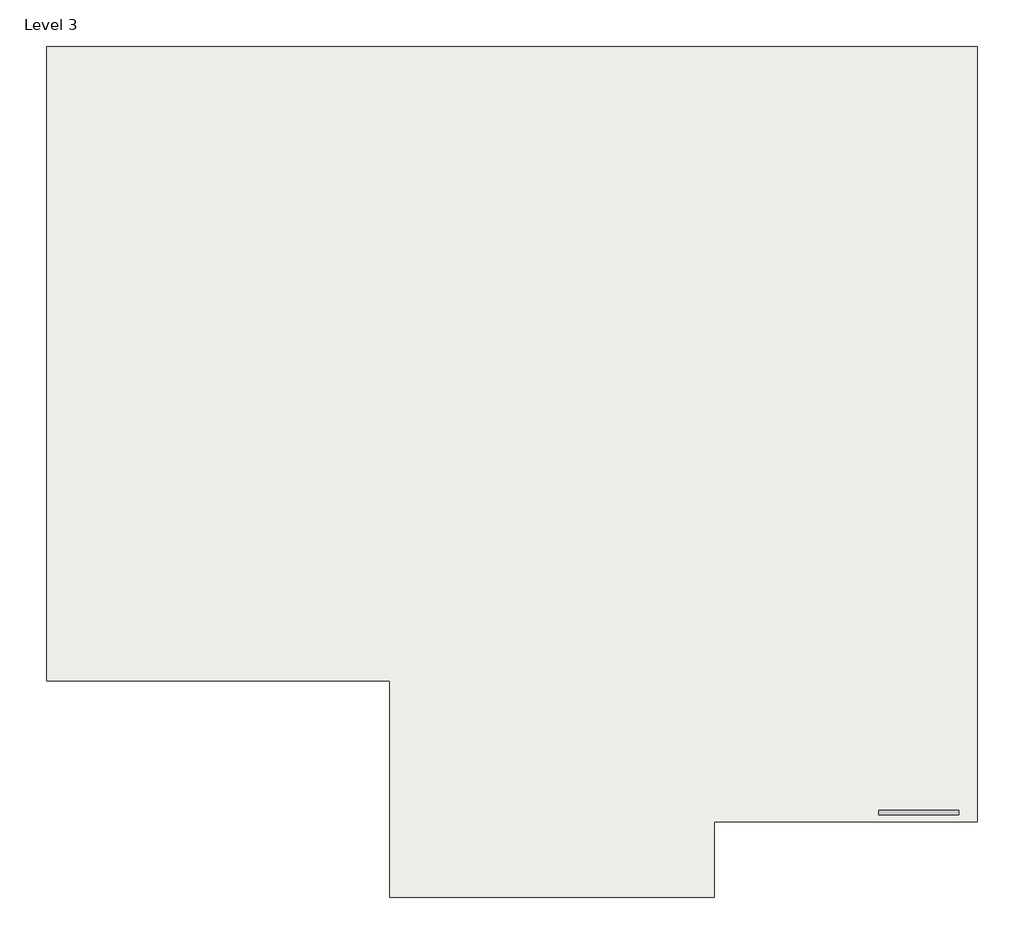
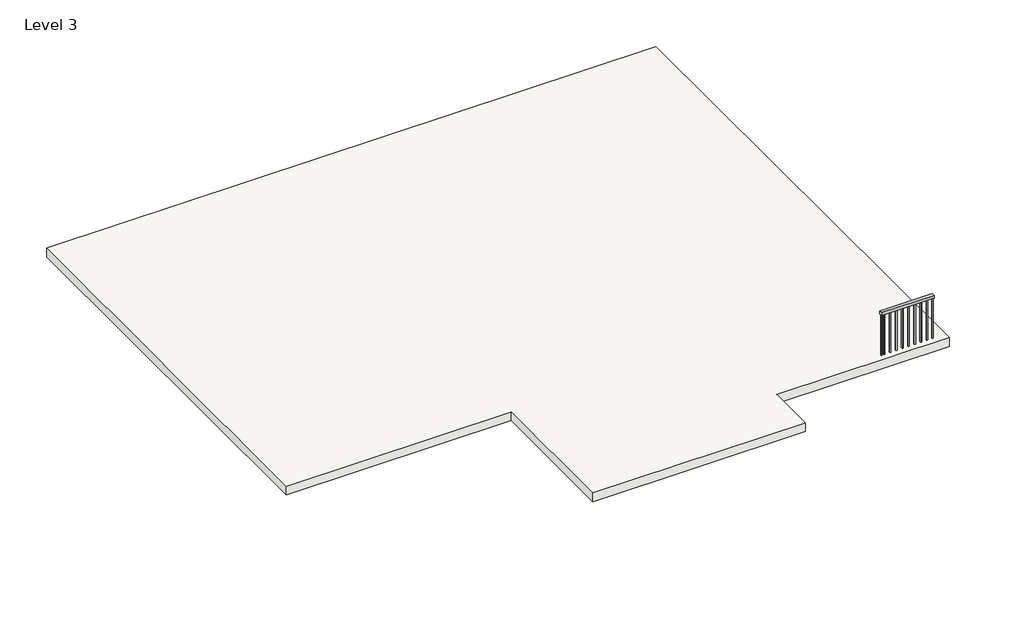
# One storey: 1 railing, 1 roof.
"""IFC4 building model written with IfcOpenShell, lengths in millimetres."""

from ifc_helpers import new_model, si_unit, frame, origin, place, context, project, spatial, polyline, outline, extrude, element, save

model = new_model("IFC4")

# Units and contexts
model_context = context("Model", 3, world=origin())
ifc_project = project(units=[si_unit("LENGTHUNIT", "METRE", prefix="MILLI")], contexts=[model_context])

# Site, building, storey
site = spatial("IfcSite", under=ifc_project)
building = spatial("IfcBuilding", under=site)
storey = spatial("IfcBuildingStorey", under=building, Name="Level 3", Elevation=3657.6)

# Railing
placement = place(None, origin())
element("IfcRailing", 1, ObjectType="Handrail - Rectangular", at=placement, inside=storey, context=model_context, shape_type="SweptSolid", body=[
    extrude(outline(polyline([(1208.040599, 5872.0433441), (1208.040599, 5821.2433441), (344.440599, 5821.2433441), (344.440599, 5872.0433441), (1208.040599, 5872.0433441)])), frame((0.0, 0.0, 4521.2), z_axis=(0.0, 0.0, 1.0), x_axis=(1.0, 0.0, 0.0)), (0.0, 0.0, 1.0), 50.8),
    extrude(outline(polyline([(404.765599, 5856.1683441), (404.765599, 5837.1183441), (385.715599, 5837.1183441), (385.715599, 5856.1683441), (404.765599, 5856.1683441)])), frame((0.0, 0.0, 3657.6), z_axis=(0.0, 0.0, 1.0), x_axis=(1.0, 0.0, 0.0)), (0.0, 0.0, 1.0), 863.6),
    extrude(outline(polyline([(506.365599, 5856.1683441), (506.365599, 5837.1183441), (487.315599, 5837.1183441), (487.315599, 5856.1683441), (506.365599, 5856.1683441)])), frame((0.0, 0.0, 3657.6), z_axis=(0.0, 0.0, 1.0), x_axis=(1.0, 0.0, 0.0)), (0.0, 0.0, 1.0), 863.6),
    extrude(outline(polyline([(607.965599, 5856.1683441), (607.965599, 5837.1183441), (588.915599, 5837.1183441), (588.915599, 5856.1683441), (607.965599, 5856.1683441)])), frame((0.0, 0.0, 3657.6), z_axis=(0.0, 0.0, 1.0), x_axis=(1.0, 0.0, 0.0)), (0.0, 0.0, 1.0), 863.6),
    extrude(outline(polyline([(709.565599, 5856.1683441), (709.565599, 5837.1183441), (690.515599, 5837.1183441), (690.515599, 5856.1683441), (709.565599, 5856.1683441)])), frame((0.0, 0.0, 3657.6), z_axis=(0.0, 0.0, 1.0), x_axis=(1.0, 0.0, 0.0)), (0.0, 0.0, 1.0), 863.6),
    extrude(outline(polyline([(811.165599, 5856.1683441), (811.165599, 5837.1183441), (792.115599, 5837.1183441), (792.115599, 5856.1683441), (811.165599, 5856.1683441)])), frame((0.0, 0.0, 3657.6), z_axis=(0.0, 0.0, 1.0), x_axis=(1.0, 0.0, 0.0)), (0.0, 0.0, 1.0), 863.6),
    extrude(outline(polyline([(912.765599, 5856.1683441), (912.765599, 5837.1183441), (893.715599, 5837.1183441), (893.715599, 5856.1683441), (912.765599, 5856.1683441)])), frame((0.0, 0.0, 3657.6), z_axis=(0.0, 0.0, 1.0), x_axis=(1.0, 0.0, 0.0)), (0.0, 0.0, 1.0), 863.6),
    extrude(outline(polyline([(1014.365599, 5856.1683441), (1014.365599, 5837.1183441), (995.315599, 5837.1183441), (995.315599, 5856.1683441), (1014.365599, 5856.1683441)])), frame((0.0, 0.0, 3657.6), z_axis=(0.0, 0.0, 1.0), x_axis=(1.0, 0.0, 0.0)), (0.0, 0.0, 1.0), 863.6),
    extrude(outline(polyline([(1115.965599, 5856.1683441), (1115.965599, 5837.1183441), (1096.915599, 5837.1183441), (1096.915599, 5856.1683441), (1115.965599, 5856.1683441)])), frame((0.0, 0.0, 3657.6), z_axis=(0.0, 0.0, 1.0), x_axis=(1.0, 0.0, 0.0)), (0.0, 0.0, 1.0), 863.6),
    extrude(outline(polyline([(363.490599, 5856.1683441), (363.490599, 5837.1183441), (344.440599, 5837.1183441), (344.440599, 5856.1683441), (363.490599, 5856.1683441)])), frame((0.0, 0.0, 3657.6), z_axis=(0.0, 0.0, 1.0), x_axis=(1.0, 0.0, 0.0)), (0.0, 0.0, 1.0), 863.6),
    extrude(outline(polyline([(1208.040599, 5856.1683441), (1208.040599, 5837.1183441), (1188.990599, 5837.1183441), (1188.990599, 5856.1683441), (1208.040599, 5856.1683441)])), frame((0.0, 0.0, 3657.6), z_axis=(0.0, 0.0, 1.0), x_axis=(1.0, 0.0, 0.0)), (0.0, 0.0, 1.0), 863.6),
])

# Roof
element("IfcRoof", 2, ObjectType="6\"", at=placement, inside=storey, context=model_context, shape_type="SweptSolid", body=[
    extrude(outline(polyline([(-8647.159401, 7269.0433441), (-8647.159401, 14127.0433441), (1411.240599, 14127.0433441), (1411.240599, 5745.0433441), (-1433.559401, 5745.0433441), (-1433.559401, 4932.2433441), (-4938.759401, 4932.2433441), (-4938.759401, 7269.0433441), (-8647.159401, 7269.0433441)])), frame((0.0, 0.0, 3657.6), z_axis=(0.0, 0.0, 1.0), x_axis=(1.0, 0.0, 0.0)), (0.0, 0.0, 1.0), 152.4),
])

save(model, "model.ifc")

# Revit data of these elements
# Type "Handrail - Rectangular"
#   Assembly Code = "C2010400"
#   built-in parameter 1008612 = 0.0416667 (stored number, unit not read)
#   built-in parameter 1008611 = 0.0416667 (stored number, unit not read)
#   built-in parameter 1008609 = 0.333333 (stored number, unit not read)
#   built-in parameter 1008604 = 0.166667 (stored number, unit not read)
#   built-in parameter 1008603 = 0.166667 (stored number, unit not read)
#   Railing Height = 3' - 0"
#   built-in parameter 1008630 = 2
#   built-in parameter 1008610 = 2
#   built-in parameter 1008618 = Baluster - Square : 3/4"
# Type "6\""
#   Assembly Code = "B1020"
#   Layers, outside or top first: 0' - 6" no material (function 1)
# Element 1 (IfcRailing, "Handrail - Rectangular")
#   Phase Created = New Construction
# Element 2 (IfcRoof, "6\"")
#   built-in parameter 1001705 = 12.5 (stored number, unit not read)
#   built-in parameter 1001710 = 33615
#   Phase Created = New Construction
#   Materials on its faces: "Default Roof"
# Materials
#   "Default Roof": colour RGB 88 101 114, transparency 0, Cost = 0
